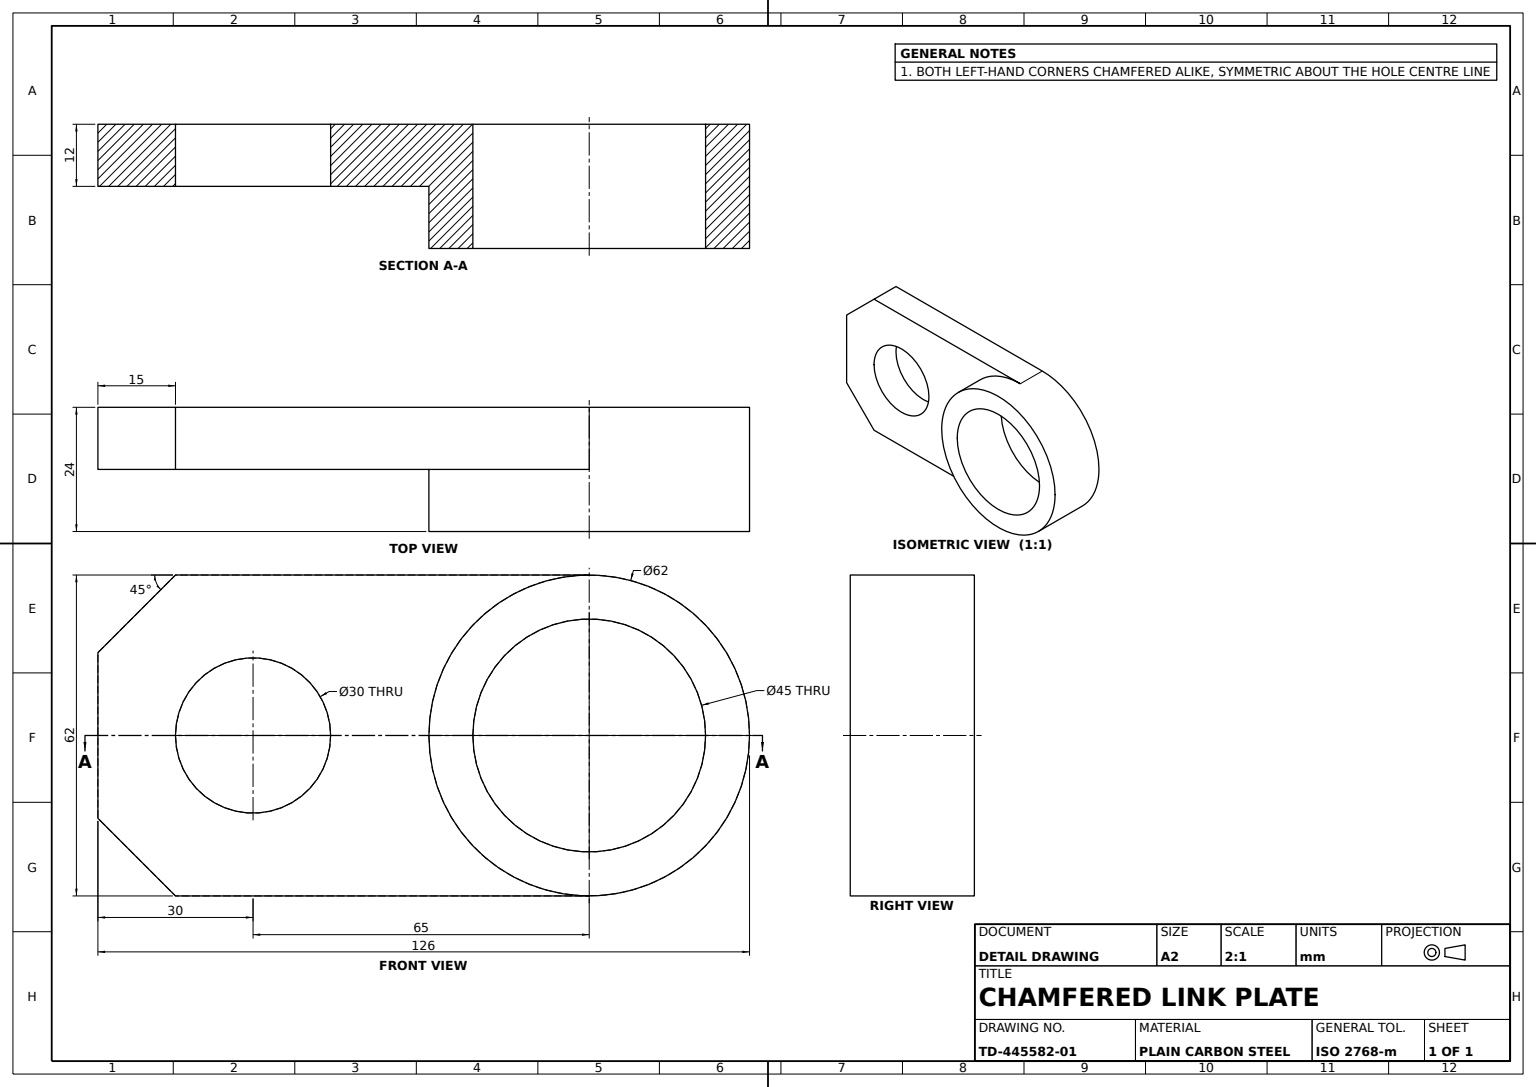
from build123d import *

# Parameters (mm, degrees)
BASE_PLATE_DEPTH = 12
BOSS_SKETCH_62_R = 31
BOSS_62_DEPTH    = 12
BORE_SKETCH_45_R = 22.5
BORE_45_DEPTH    = 25
HOLE_SKETCH_30_R = 15
HOLE_30_DEPTH    = 25


with BuildPart() as part:
    # Base Plate Sketch → Base Plate (new body)
    with BuildSketch(Plane.XY):
        with BuildLine():
            Line((-15, -31), (65, -31))
            ThreePointArc((65, -31), (96, 0), (65, 31))
            Line((65, 31), (-15, 31))
            Line((-15, 31), (-30, 16))
            Line((-30, 16), (-30, 0))
            Line((-30, 0), (-30, -16))
            Line((-30, -16), (-15, -31))
        make_face()
    extrude(amount=BASE_PLATE_DEPTH)

    # Boss Sketch Ø62 → Boss Ø62 (add)
    with BuildSketch(Plane.XY.offset(12)):
        with Locations(Location((65, 0, 0), (0, 0, 90))):
            Circle(BOSS_SKETCH_62_R)
    extrude(amount=BOSS_62_DEPTH)

    # Bore Sketch Ø45 → Bore Ø45 (cut)
    with BuildSketch(Plane.XY.offset(24)):
        with Locations((65, 0)):
            Circle(BORE_SKETCH_45_R)
    extrude(amount=-BORE_45_DEPTH, mode=Mode.SUBTRACT)

    # Hole Sketch Ø30 → Hole Ø30 (cut)
    with BuildSketch(Plane.XY.offset(12)):
        Circle(HOLE_SKETCH_30_R)
    extrude(amount=-HOLE_30_DEPTH, mode=Mode.SUBTRACT)


solid = part.part
